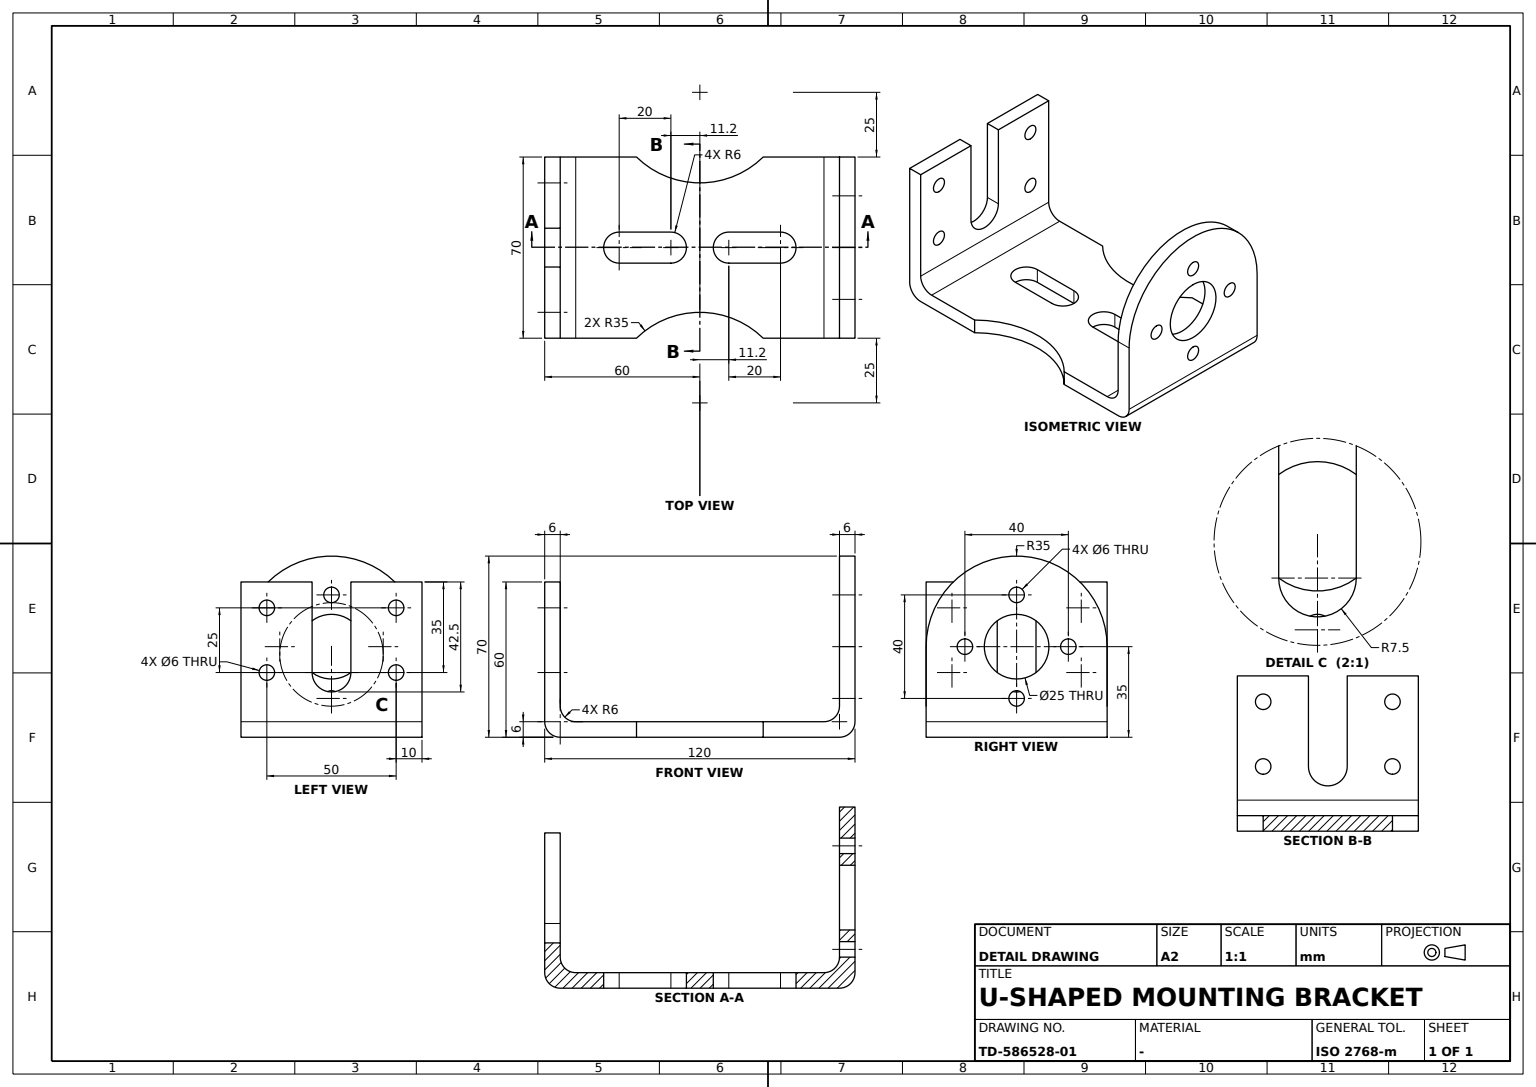
CATIA V5 part; units mm, degrees
sketch "Sketch1" plane through (0, 0, 0) normal (0, 0, 1) x (0, 1, 0)
  line L0 (0, 0) -> (35.5051, 0)
  line L1 (120, 0) -> (120, -70)
  line L2 (120, -70) -> (84.4949, -70)
  line L3 (0, -70) -> (0, 0)
  point P0 (120, -70)
  point P1 (0, -70)
  arc A0 (84.4949, -70) -> (35.5051, -70) centre (60, -95) ccw
  point P2 (60, -95)
  point P3 (35.5051, -70)
  line L4 (35.5051, -70) -> (0, -70)
  arc A1 (84.4949, 0) -> (35.5051, 0) centre (60, 25) cw
  line L5 (84.4949, 0) -> (120, 0)
  dimension "length L1" = 70
  dimension "radius A0" = 35
  dimension "distance P2 L3" = 60
  dimension "distance A0 L2" = 10
  dimension "distance P0 P1" = 120
  constraint horizontal L0 x-axis
  constraint horizontal L2 x-axis
  constraint horizontal L4 x-axis
  constraint horizontal L5 x-axis
  constraint vertical L1 y-axis
  constraint vertical L3 y-axis
  constraint coincidence L2 P3
  constraint coincidence L2 L4
  constraint coincidence L0 L5
extrude "Pad1" add sketch "Sketch1" along normal blind 6
sketch "Sketch2" plane through (0, 120, 0) normal (0, 1, 0) x (-1, 0, 0)
  point P0 (-35, 35)
  line L0 (-70, 5.2447) -> (-70, 35)
  line L1 (0, 5.2447) -> (0, 35)
  arc A0 (0, 35) -> (-70, 35) centre (-35, 35) ccw
  line L2 (-70, 5.2447) -> (0, 5.2447)
  dimension "D1" = 35
  constraint horizontal L2 x-axis
extrude "Pad2" add sketch "Sketch2" against normal blind 6
sketch "Sketch3" plane through (0, 0, 0) normal (0, -1, 0) x (1, 0, 0)
  line L0 (0, 0) -> (70, 0)
  line L1 (70, 0) -> (70, 60)
  line L2 (70, 60) -> (0, 60)
  line L3 (0, 60) -> (0, 0)
  dimension "length L1" = 60
  dimension "length L2" = 70
  constraint horizontal L0 x-axis
  constraint horizontal L2 x-axis
  constraint vertical L1 y-axis
  constraint vertical L3 y-axis
extrude "Pad3" add sketch "Sketch3" against normal blind 6
sketch "Sketch4" plane through (0, 0, 0) normal (0, -1, 0) x (1, 0, 0)
  arc A0 (27.5, 25) -> (42.5, 25) centre (35, 25) ccw
  point P0 (35, 25)
  line L0 (70, 60) -> (0, 60) construction
  line L1 (27.5, 25) -> (27.5, 60.1785)
  point P1 (27.5, 25)
  point P2 (42.5, 25)
  line L2 (42.5, 25) -> (42.5, 60.1785)
  line L3 (27.5, 60.1785) -> (42.5, 60.1785)
  point P3 (27.5, 25)
  point P4 (42.5, 25)
  dimension "radius A0" = 7.5
  dimension "distance P0 L0" = 35
  constraint coincidence P1 A0
  constraint coincidence L2 P4
  constraint coincidence L1 P3
  constraint coincidence P1 P3
  constraint coincidence P2 P4
  constraint tangency L1 A0
  constraint horizontal L3 x-axis
extrude "Pocket1" cut sketch "Sketch4" against normal blind 6
fillet "Fillet1" radius 6 4 edges at (35, 120, 0) (35, 6, 6) (35, 114, 6) (35, 0, 0)
sketch "Sketch5" plane through (33.8606, 120, 52.2904) normal (0, 1, 0) x (1, 0, 0)
  point P0 (1.1394, 17.2904)
  arc A0 (-33.8606, 17.2904) -> (36.1394, 17.2904) centre (1.1394, 17.2904) ccw construction
  constraint concentricity A0 P0
hole "Hole1" at (35, 120, 35) direction (0, -1, 0) diameter 25 end up to next
sketch "Sketch6" plane through (0, 120, 0) normal (0, 1, 0) x (-1, 0, 0)
  circle A0 centre (-35, 35) radius 20 construction
  point P0 (-35, 35)
  circle A1 centre (-35, 55) radius 3
  point P1 (-35, 55)
  circle A2 centre (-55, 35) radius 3
  point P2 (-55, 35)
  circle A3 centre (-15, 35) radius 3
  point P3 (-15, 35)
  circle A4 centre (-35, 15) radius 3
  point P4 (-35, 15)
  dimension "radius A0" = 20
  dimension "D2" = 35
  dimension "D3" = 35
  dimension "radius A1" = 3
  dimension "radius A2" = 3
  dimension "radius A3" = 3
  dimension "radius A4" = 3
  constraint coincidence P1 A0
  constraint coincidence P2 A0
  constraint coincidence P3 A0
  constraint coincidence P4 A0
extrude "Pocket2" cut sketch "Sketch6" against normal up to next
sketch "Sketch7" plane through (0, 0, 0) normal (0, -1, 0) x (1, 0, 0)
  circle A0 centre (10, 50) radius 3
  point P0 (10, 50)
  line L0 (0, 6) -> (0, 0) construction
  circle A1 centre (10, 25) radius 3
  point P1 (10, 25)
  line L1 (70, 60) -> (0, 60) construction
  circle A2 centre (60, 50) radius 3
  circle A3 centre (60, 25) radius 3
  dimension "radius A0" = 3
  dimension "distance P0 L0" = 10
  dimension "radius A1" = 3
  dimension "distance P1 L1" = 35
  dimension "distance P1 P0" = 25
extrude "Pocket3" cut sketch "Sketch7" against normal up to next
sketch "Sketch8" plane through (0, 0, 6) normal (0, 0, 1) x (0, 1, 0)
  line L0 (60, -22.9842) -> (60, -47.6343) construction
  line L1 (120, 0) -> (120, -70) construction
  line L2 (50.3956, -35) -> (68.97, -35) construction
  line L3 (0, -70) -> (35.5051, -70) construction
  line L4 (28.8035, -35) -> (48.8035, -35) construction
  point P0 (28.8035, -35)
  point P1 (48.8035, -35)
  line L5 (28.8035, -29) -> (48.8035, -29)
  line L6 (48.8035, -41) -> (28.8035, -41)
  arc A0 (48.8035, -29) -> (48.8035, -41) centre (48.8035, -35) cw
  arc A1 (28.8035, -41) -> (28.8035, -29) centre (28.8035, -35) cw
  point P2 (28.8035, -29)
  point P3 (48.8035, -29)
  point P4 (48.8035, -41)
  point P5 (28.8035, -41)
  point P6 (71.1965, -29)
  point P7 (91.1965, -29)
  line L7 (91.1965, -29) -> (71.1965, -29)
  point P8 (91.1965, -41)
  point P9 (71.1965, -41)
  line L8 (71.1965, -41) -> (91.1965, -41)
  arc A2 (71.1965, -29) -> (71.1965, -41) centre (71.1965, -35) ccw
  arc A3 (91.1965, -41) -> (91.1965, -29) centre (91.1965, -35) ccw
  dimension "distance L0 L1" = 60
  dimension "distance L2 L3" = 35
  dimension "distance L4 L5" = 6
  dimension "distance P1 P0" = 20
  dimension "distance P1 L0" = 11.1965
  constraint vertical L0 y-axis
  constraint horizontal L2 x-axis
  constraint horizontal L4 x-axis
  constraint coincidence P0 L2
  constraint tangency A0 L5
  constraint tangency A1 L5
  constraint tangency A0 L6
  constraint tangency A1 L6
  constraint symmetry P3 P6 L0
  constraint symmetry P2 P7 L0
  constraint symmetry L5 L7 L0
  constraint symmetry P5 P8 L0
  constraint symmetry P4 P9 L0
  constraint symmetry L6 L8 L0
  constraint symmetry A0 A2 L0
  constraint symmetry A1 A3 L0
extrude "Pocket4" cut sketch "Sketch8" against normal up to next
properties part number "catia 20"
